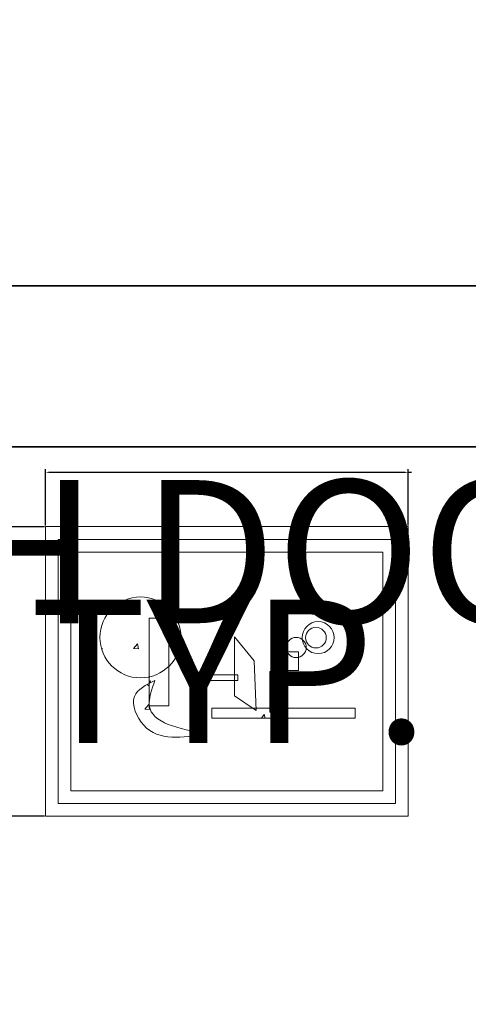
# Model space of a CAD drawing. Units: inches. Extents: x 125 to 976, y 231 to 853.
# Tile 6 of 16: x 393 to 418, y 463 to 518. Entities that reach past the tile are written whole.
import ezdxf

# ---------------------------------------------------------------- set-up
doc = ezdxf.new("R2010")
doc.units = ezdxf.units.IN
doc.header["$MEASUREMENT"] = 0
for name, color, linetype, lineweight in [('A-ANNO-DIMS', 2, 'Continuous', 18), ('A-FURN-ARTW', 9, 'Continuous', 13), ('A-WALL', 7, 'Continuous', 35)]:
    doc.layers.add(name, color=color, linetype=linetype, lineweight=lineweight)
doc.styles.get("Standard").update_dxf_attribs({"font": 'italic8.shx'})
doc.dimstyles.get("Standard").update_dxf_attribs({"dimtxt": 8, "dimasz": 0.18, "dimexe": 0.18, "dimexo": 0.0625, "dimgap": 0.09, "dimtad": 0, "dimtih": 1, "dimtoh": 1, "dimdec": 4, "dimzin": 0, "dimdsep": 46, "dimlunit": 3, "dimtxsty": 'Standard', "dimcen": 0.09, "dimclrt": 4, "dimadec": 0, "dimazin": 0, "dimtfac": 1, "dimtdec": 4, "dimtofl": 0, "dimtmove": 0, "dimatfit": 3, "dimfxl": 1, "dimtolj": 1, "dimtzin": 0, "dimarcsym": 0})

# ---------------------------------------------------------------- blocks, each defined once
blk = doc.blocks.new('ART-FRAMED-ABSTRACT')
for p, q in [((-0.001, 16.177), (20.24, 16.177)), ((-0.001, 0.003), (-0.001, 16.177)), ((20.24, 16.177), (20.24, 0.003)), ((0.708, 15.468), (19.531, 15.468)), ((0.708, 0.712), (0.708, 15.468)), ((0.708, 15.468), (19.531, 15.468)), ((0.708, 0.712), (0.708, 15.468)), ((19.531, 15.468), (19.531, 0.712)), ((19.531, 15.468), (19.531, 0.712)), ((1.416, 14.76), (18.823, 14.76)), ((1.416, 1.421), (1.416, 14.76)), ((18.823, 14.76), (18.823, 1.421)), ((5.788, 11.063), (6.882, 11.063)), ((5.788, 6.173), (5.788, 11.063)), ((6.882, 11.063), (6.882, 6.173)), ((6.882, 10.801), (6.949, 10.827)), ((6.882, 10.625), (6.95, 10.826)), ((10.548, 10.016), (11.64, 8.68)), ((10.548, 6.716), (10.548, 10.016)), ((3.124, 9.359), (3.168, 9.375)), ((3.143, 9.298), (3.169, 9.375)), ((4.91, 9.372), (5.178, 9.348)), ((4.911, 9.372), (5.128, 9.631)), ((5.182, 9.343), (5.13, 9.625)), ((13.432, 8.139), (13.432, 9.18)), ((13.432, 9.18), (14.107, 9.18)), ((14.107, 9.18), (14.107, 8.139)), ((11.64, 8.68), (11.749, 5.898)), ((8.712, 7.894), (10.735, 7.894)), ((8.712, 7.588), (8.712, 7.894)), ((10.735, 7.894), (10.735, 7.588)), ((12.758, 8.078), (12.513, 8.078)), ((12.513, 8.078), (12.513, 5.812)), ((12.758, 5.812), (12.758, 8.078)), ((14.107, 8.139), (13.432, 8.139)), ((5.664, 7.358), (5.763, 7.291)), ((5.764, 7.291), (5.788, 7.365)), ((5.788, 7.538), (5.854, 7.564)), ((5.812, 7.436), (5.855, 7.563)), ((10.735, 7.588), (8.712, 7.588)), ((11.749, 5.898), (10.548, 6.716)), ((5.535, 5.988), (5.752, 6.246)), ((5.806, 5.958), (5.754, 6.241)), ((6.882, 6.173), (5.788, 6.173)), ((5.534, 5.987), (5.803, 5.964)), ((17.282, 6.043), (9.282, 6.043)), ((9.282, 6.043), (9.282, 5.486)), ((12.044, 5.486), (12.207, 5.681)), ((12.244, 5.486), (12.209, 5.676)), ((12.513, 5.812), (12.758, 5.812)), ((17.282, 5.486), (17.282, 6.043)), ((9.282, 5.486), (17.282, 5.486)), ((18.823, 1.421), (1.416, 1.421)), ((19.531, 0.712), (0.708, 0.712)), ((19.531, 0.712), (0.708, 0.712)), ((20.24, 0.003), (-0.001, 0.003))]:
    blk.add_line(p, q)
for centre, radius in [((5.295, 9.99), 2.26), ((15.21, 9.976), 0.893), ((15.088, 9.976), 0.578), ((13.984, 9.425), 0.565)]:
    blk.add_circle(centre, radius)
for points, knots in [([(6.101, 7.577), (5.604, 7.338), (4.526, 6.817), (5.68, 4.068), (7.637, 4.378), (8.957, 4.588)], [0, 0, 0, 0, 1.44737, 3.141992, 6.657621, 6.657621, 6.657621, 6.657621]), ([(6.101, 7.577), (5.92, 7.073), (5.293, 5.325), (7.434, 4.894), (8.957, 4.588)], [0, 0, 0, 0, 1.438871, 4.981716, 4.981716, 4.981716, 4.981716])]:
    blk.add_open_spline(points, degree=3, knots=knots)
blk = doc.blocks.new('*D40')
at = {"layer": 'A-ANNO-DIMS', "color": 0, "lineweight": -2, "transparency": 16777216}
for p, q in [((322.587, 494.042), (322.587, 488.075)), ((361.587, 494.042), (361.587, 488.075)), ((322.767, 488.255), (361.407, 488.255)), ((361.587, 488.255), (361.767, 488.255))]:
    blk.add_line(p, q, dxfattribs=at)
at = {"layer": 'A-ANNO-DIMS', "color": 0, "transparency": 16777216}
for points in [[(322.767, 488.285), (322.767, 488.225), (322.587, 488.255)], [(361.407, 488.285), (361.407, 488.225), (361.587, 488.255)]]:
    blk.add_solid(points, dxfattribs=at)
at = {"layer": 'Defpoints', "color": 0, "transparency": 16777216}
for p in [(322.587, 494.105), (361.587, 494.105), (361.587, 488.255)]:
    blk.add_point(p, dxfattribs=at)
at = {"layer": 'A-ANNO-DIMS', "color": 4, "transparency": 16777216, "insert": (432.523, 488.255), "char_height": 8, "attachment_point": 5}
blk.add_mtext('\\A1;RH DOOR 3\'-3" TYP.', dxfattribs=at)
blk = doc.blocks.new('*D44')
at = {"layer": 'A-ANNO-DIMS', "color": 0, "lineweight": -2, "transparency": 16777216}
for p, q in [((394.866, 489.715), (394.866, 492.869)), ((395.046, 492.689), (414.927, 492.689)), ((415.107, 489.715), (415.107, 492.869)), ((415.107, 492.689), (415.287, 492.689))]:
    blk.add_line(p, q, dxfattribs=at)
at = {"layer": 'A-ANNO-DIMS', "color": 0, "transparency": 16777216}
for points in [[(395.046, 492.719), (395.046, 492.659), (394.866, 492.689)], [(414.927, 492.719), (414.927, 492.659), (415.107, 492.689)]]:
    blk.add_solid(points, dxfattribs=at)
at = {"layer": 'Defpoints', "color": 0, "transparency": 16777216}
for p in [(415.107, 492.689), (394.866, 489.652), (415.107, 489.652)]:
    blk.add_point(p, dxfattribs=at)
at = {"layer": 'A-ANNO-DIMS', "color": 4, "transparency": 16777216, "insert": (498.425, 492.689), "char_height": 8, "attachment_point": 5}
blk.add_mtext('\\A1;FRAMED ART 1\'-8" TYP.', dxfattribs=at)
blk = doc.blocks.new('*D45')
at = {"layer": 'A-ANNO-DIMS', "color": 0, "lineweight": -2, "transparency": 16777216}
for p, q in [((394.804, 489.652), (391.65, 489.652)), ((391.83, 489.472), (391.83, 486.418)), ((391.83, 473.659), (391.83, 476.714)), ((394.804, 473.479), (391.65, 473.479))]:
    blk.add_line(p, q, dxfattribs=at)
at = {"layer": 'A-ANNO-DIMS', "color": 0, "transparency": 16777216}
for points in [[(391.8, 489.472), (391.86, 489.472), (391.83, 489.652)], [(391.8, 473.659), (391.86, 473.659), (391.83, 473.479)]]:
    blk.add_solid(points, dxfattribs=at)
at = {"layer": 'Defpoints', "color": 0, "transparency": 16777216}
for p in [(391.83, 489.652), (394.866, 489.652), (394.866, 473.479)]:
    blk.add_point(p, dxfattribs=at)
at = {"layer": 'A-ANNO-DIMS', "color": 4, "transparency": 16777216, "insert": (391.83, 481.566), "char_height": 8, "attachment_point": 5}
blk.add_mtext('\\A1;1\'-4" TYP.', dxfattribs=at)

msp = doc.modelspace()

# ---------------------------------------------------------------- linework, layer by layer
at = {"layer": 'A-WALL'}
for p, q in [((372.5792, 503.10475), (456.5792, 503.10475)), ((361.58656, 494.10475), (456.5792, 494.10475))]:
    msp.add_line(p, q, dxfattribs=at)

# ---------------------------------------------------------------- block references
at = {"layer": 'A-FURN-ARTW'}
msp.add_blockref('ART-FRAMED-ABSTRACT', (394.86728, 473.47531), dxfattribs=at)

# ---------------------------------------------------------------- dimensions: what is measured, and where the dimension line sits
at = {"layer": 'A-ANNO-DIMS'}
for base, p1, p2, text, picture, middle in [((415.10718, 492.68858), (394.86616, 489.65243), (415.10718, 489.65243), 'FRAMED ART <> TYP.', '*D44', (498.4248, 492.68858)), ((361.58656, 488.25475), (322.58656, 494.10475), (361.58656, 494.10475), 'RH DOOR <> TYP.', '*D40', (432.52323, 488.25475))]:
    dim = msp.add_linear_dim(base=base, p1=p1, p2=p2, text=text, dimstyle='Standard', override={"dimdec": 1, "dimlfac": 1, "dimrnd": 0, "dimzin": 1, "dimdsep": 46, "dimlunit": 4, "dimfrac": 2}, dxfattribs=at)
    dim.commit()
    dim.dimension.update_dxf_attribs({"geometry": picture, "text_midpoint": middle})
dim = msp.add_linear_dim(base=(391.83, 489.65243), p1=(394.86616, 473.47878), p2=(394.86616, 489.65243), angle=90, text='<> TYP.', dimstyle='Standard', override={"dimdec": 1, "dimlfac": 1, "dimrnd": 0, "dimzin": 1, "dimdsep": 46, "dimlunit": 4, "dimfrac": 2}, dxfattribs=at)
dim.commit()
dim.dimension.update_dxf_attribs({"geometry": '*D45', "text_midpoint": (391.83, 481.5656)})

doc.saveas('drawing.dxf')
